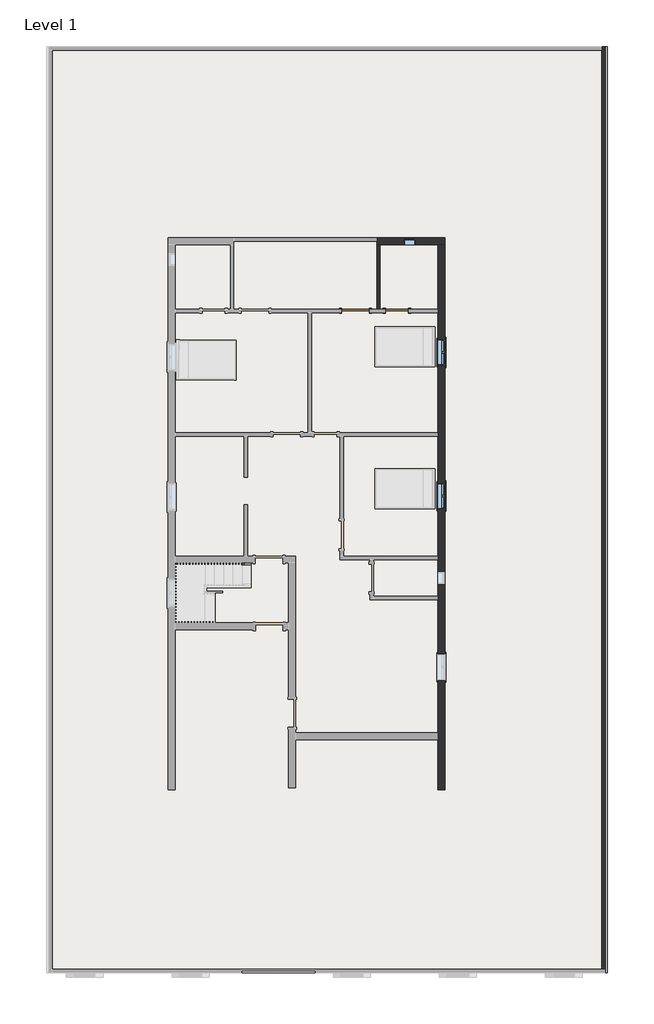
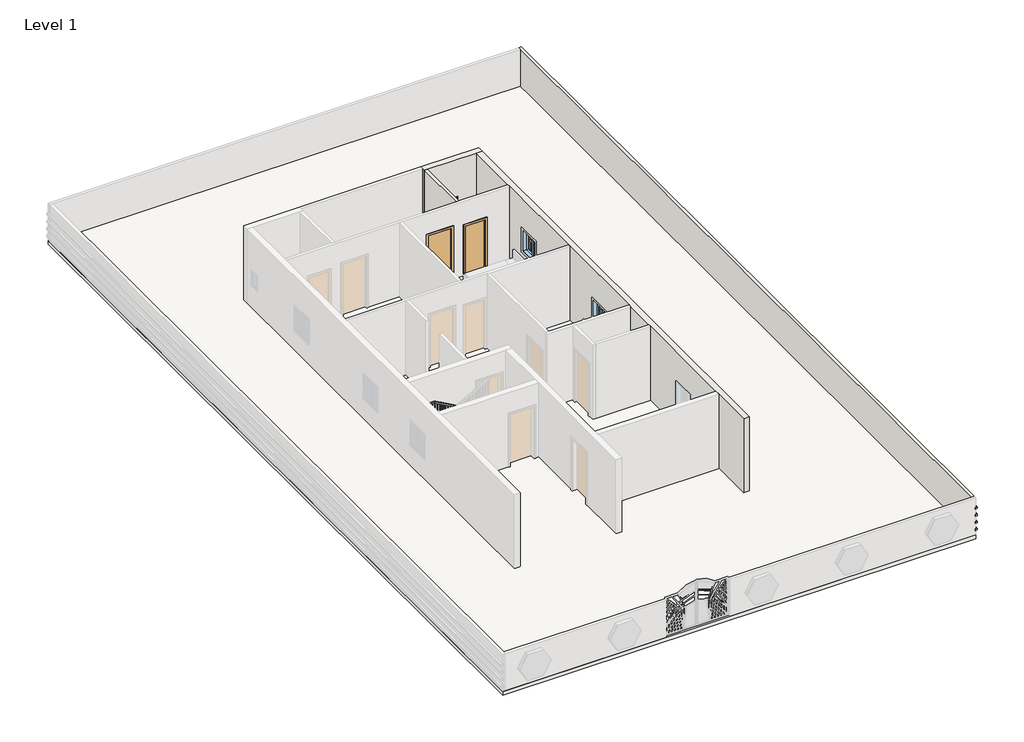
# One storey, part 2 of 3: 4 proxies, 4 walls, 3 windows, 2 doors, 1 railing, 1 slab.
"""IFC4 building model written with IfcOpenShell, lengths in millimetres."""

from ifc_helpers import new_model, si_unit, frame, origin, origin_with_axes, place, context, project, spatial, polyline, outline, extrude, faceted_brep, transform, mapped, element, save
from components import door_f2b275c1, door_e5f9f3c4, window_aa618e30, window_339605e1

model = new_model("IFC4")

# Units and contexts
model_context = context("Model", 3, world=origin())
ifc_project = project(units=[si_unit("LENGTHUNIT", "METRE", prefix="MILLI")], contexts=[model_context])

# Site, building, storey
site = spatial("IfcSite", under=ifc_project)
building = spatial("IfcBuilding", under=site)
storey = spatial("IfcBuildingStorey", under=building, Name="Level 1", Elevation=0.0)

# Proxies
placement = place(None, origin())
element("IfcBuildingElementProxy", 1, Name="Reveal", ObjectType="Reveal", at=placement, inside=storey, context=model_context, shape_type="SweptSolid", body=[
    extrude(outline(polyline([(8597.0265354, 16740.4715095), (8689.1015354, 16740.4715095), (8689.1015354, -13853.8284905), (8597.0265354, -13853.8284905), (8597.0265354, 16740.4715095)])), frame((0.0, 0.0, 1066.8), z_axis=(0.0, 0.0, 1.0), x_axis=(1.0, 0.0, 0.0)), (0.0, 0.0, 1.0), 67.7333333),
])
element("IfcBuildingElementProxy", 2, Name="Reveal", ObjectType="Reveal", at=placement, inside=storey, context=model_context, shape_type="SweptSolid", body=[
    extrude(outline(polyline([(8597.0265354, 16740.4715095), (8689.1015354, 16740.4715095), (8689.1015354, -13853.8284905), (8597.0265354, -13853.8284905), (8597.0265354, 16740.4715095)])), frame((0.0, 0.0, 772.755123), z_axis=(0.0, 0.0, 1.0), x_axis=(1.0, 0.0, 0.0)), (0.0, 0.0, 1.0), 67.7333333),
])
element("IfcBuildingElementProxy", 3, Name="Reveal", ObjectType="Reveal", at=placement, inside=storey, context=model_context, shape_type="SweptSolid", body=[
    extrude(outline(polyline([(8597.0265354, 16740.4715095), (8689.1015354, 16740.4715095), (8689.1015354, -13853.8284905), (8597.0265354, -13853.8284905), (8597.0265354, 16740.4715095)])), frame((0.0, 0.0, 478.710246), z_axis=(0.0, 0.0, 1.0), x_axis=(1.0, 0.0, 0.0)), (0.0, 0.0, 1.0), 67.7333333),
])
element("IfcBuildingElementProxy", 4, Name="Reveal", ObjectType="Reveal", at=placement, inside=storey, context=model_context, shape_type="SweptSolid", body=[
    extrude(outline(polyline([(8597.0265354, 16740.4715095), (8689.1015354, 16740.4715095), (8689.1015354, -13853.8284905), (8597.0265354, -13853.8284905), (8597.0265354, 16740.4715095)])), frame((0.0, 0.0, 184.6653689), z_axis=(0.0, 0.0, 1.0), x_axis=(1.0, 0.0, 0.0)), (0.0, 0.0, 1.0), 67.7333333),
])

# Doors
door_shape = door_f2b275c1(model_context)
element("IfcDoor", 5, ObjectType="Single-Flush : 30\" x 80\"", at=placement, inside=storey, context=model_context, shape_type="MappedRepresentation", body=[
    mapped(door_shape, transform((1735.6084916, 8007.7072267, 0.0), x_axis=(-1.0, 0.0, 0.0), y_axis=(0.0, -1.0, 0.0), z_axis=(0.0, 0.0, 1.0))),
])
door_2_shape = door_e5f9f3c4(model_context)
element("IfcDoor", 6, ObjectType="Single-Flush : 36\" x 84\"", at=placement, inside=storey, context=model_context, shape_type="MappedRepresentation", body=[
    mapped(door_2_shape, transform((364.0084916, 8007.7072267, 0.0), x_axis=(1.0, 0.0, 0.0), y_axis=(0.0, 1.0, 0.0), z_axis=(0.0, 0.0, 1.0))),
])

# Railing
element("IfcRailing", 7, ObjectType="Handrail - Rectangular", at=placement, inside=storey, context=model_context, shape_type="SolidModel", body=[
    faceted_brep([(-3084.0415084, -367.9427733, 1083.7333333), (-3084.0415084, -367.9427733, 1025.620221), (-3084.0415084, -317.1427733, 1025.620221), (-3084.0415084, -317.1427733, 1083.7333333), (-4608.0415084, -367.9427733, 1930.4), (-4621.2051106, -367.9427733, 1879.6), (-4621.2051106, -317.1427733, 1879.6), (-4608.0415084, -317.1427733, 1930.4), (-5547.8415084, -367.9427733, 1930.4), (-5547.8415084, -367.9427733, 1879.6), (-5598.6415084, -317.1427733, 1879.6), (-5598.6415084, -317.1427733, 1930.4), (-5547.8415084, -2247.5427733, 1930.4), (-5547.8415084, -2247.5427733, 1879.6), (-5598.6415084, -2298.3427733, 1879.6), (-5598.6415084, -2298.3427733, 1930.4), (-4912.8415084, -2247.5427733, 1930.4), (-4899.6779062, -2247.5427733, 1879.6), (-4899.6779062, -2298.3427733, 1879.6), (-4912.8415084, -2298.3427733, 1930.4), (-3084.0415084, -2247.5427733, 2946.4), (-3084.0415084, -2298.3427733, 2946.4), (-3084.0415084, -2298.3427733, 2888.2868876), (-3084.0415084, -2247.5427733, 2888.2868876)], [[[0, 1, 2, 3]], [[1, 0, 4, 5]], [[2, 1, 5, 6]], [[3, 2, 6, 7]], [[0, 3, 7, 4]], [[5, 4, 8, 9]], [[6, 5, 9, 10]], [[7, 6, 10, 11]], [[4, 7, 11, 8]], [[9, 8, 12, 13]], [[10, 9, 13, 14]], [[11, 10, 14, 15]], [[8, 11, 15, 12]], [[13, 12, 16, 17]], [[14, 13, 17, 18]], [[15, 14, 18, 19]], [[12, 15, 19, 16]], [[20, 21, 22, 23]], [[17, 16, 20, 23]], [[18, 17, 23, 22]], [[19, 18, 22, 21]], [[16, 19, 21, 20]]]),
    extrude(outline(polyline([(2865.3563321, -3125.3165084), (2854.7729988, -3144.3665084), (1862.6666667, -3144.3665084), (1862.6666667, -3125.3165084), (2865.3563321, -3125.3165084)])), frame((0.0, -2282.4677733, 0.0), z_axis=(0.0, 1.0, 0.0), x_axis=(0.0, 0.0, 1.0)), (0.0, 0.0, 1.0), 19.05),
    extrude(outline(polyline([(2808.9118876, -3226.9165084), (2798.3285543, -3245.9665084), (1862.6666667, -3245.9665084), (1862.6666667, -3226.9165084), (2808.9118876, -3226.9165084)])), frame((0.0, -2282.4677733, 0.0), z_axis=(0.0, 1.0, 0.0), x_axis=(0.0, 0.0, 1.0)), (0.0, 0.0, 1.0), 19.05),
    extrude(outline(polyline([(2752.4674432, -3328.5165084), (2741.8841099, -3347.5665084), (1862.6666667, -3347.5665084), (1862.6666667, -3328.5165084), (2752.4674432, -3328.5165084)])), frame((0.0, -2282.4677733, 0.0), z_axis=(0.0, 1.0, 0.0), x_axis=(0.0, 0.0, 1.0)), (0.0, 0.0, 1.0), 19.05),
    extrude(outline(polyline([(2696.0229988, -3430.1165084), (2685.4396654, -3449.1665084), (1693.3333333, -3449.1665084), (1693.3333333, -3430.1165084), (2696.0229988, -3430.1165084)])), frame((0.0, -2282.4677733, 0.0), z_axis=(0.0, 1.0, 0.0), x_axis=(0.0, 0.0, 1.0)), (0.0, 0.0, 1.0), 19.05),
    extrude(outline(polyline([(2639.5785543, -3531.7165084), (2628.995221, -3550.7665084), (1693.3333333, -3550.7665084), (1693.3333333, -3531.7165084), (2639.5785543, -3531.7165084)])), frame((0.0, -2282.4677733, 0.0), z_axis=(0.0, 1.0, 0.0), x_axis=(0.0, 0.0, 1.0)), (0.0, 0.0, 1.0), 19.05),
    extrude(outline(polyline([(2583.1341099, -3633.3165084), (2572.5507765, -3652.3665084), (1693.3333333, -3652.3665084), (1693.3333333, -3633.3165084), (2583.1341099, -3633.3165084)])), frame((0.0, -2282.4677733, 0.0), z_axis=(0.0, 1.0, 0.0), x_axis=(0.0, 0.0, 1.0)), (0.0, 0.0, 1.0), 19.05),
    extrude(outline(polyline([(2526.6896654, -3734.9165084), (2516.1063321, -3753.9665084), (1524.0, -3753.9665084), (1524.0, -3734.9165084), (2526.6896654, -3734.9165084)])), frame((0.0, -2282.4677733, 0.0), z_axis=(0.0, 1.0, 0.0), x_axis=(0.0, 0.0, 1.0)), (0.0, 0.0, 1.0), 19.05),
    extrude(outline(polyline([(2470.245221, -3836.5165084), (2459.6618876, -3855.5665084), (1524.0, -3855.5665084), (1524.0, -3836.5165084), (2470.245221, -3836.5165084)])), frame((0.0, -2282.4677733, 0.0), z_axis=(0.0, 1.0, 0.0), x_axis=(0.0, 0.0, 1.0)), (0.0, 0.0, 1.0), 19.05),
    extrude(outline(polyline([(2413.8007765, -3938.1165084), (2403.2174432, -3957.1665084), (1524.0, -3957.1665084), (1524.0, -3938.1165084), (2413.8007765, -3938.1165084)])), frame((0.0, -2282.4677733, 0.0), z_axis=(0.0, 1.0, 0.0), x_axis=(0.0, 0.0, 1.0)), (0.0, 0.0, 1.0), 19.05),
    extrude(outline(polyline([(2357.3563321, -4039.7165084), (2346.7729988, -4058.7665084), (1354.6666667, -4058.7665084), (1354.6666667, -4039.7165084), (2357.3563321, -4039.7165084)])), frame((0.0, -2282.4677733, 0.0), z_axis=(0.0, 1.0, 0.0), x_axis=(0.0, 0.0, 1.0)), (0.0, 0.0, 1.0), 19.05),
    extrude(outline(polyline([(2300.9118876, -4141.3165084), (2290.3285543, -4160.3665084), (1354.6666667, -4160.3665084), (1354.6666667, -4141.3165084), (2300.9118876, -4141.3165084)])), frame((0.0, -2282.4677733, 0.0), z_axis=(0.0, 1.0, 0.0), x_axis=(0.0, 0.0, 1.0)), (0.0, 0.0, 1.0), 19.05),
    extrude(outline(polyline([(2244.4674432, -4242.9165084), (2233.8841099, -4261.9665084), (1354.6666667, -4261.9665084), (1354.6666667, -4242.9165084), (2244.4674432, -4242.9165084)])), frame((0.0, -2282.4677733, 0.0), z_axis=(0.0, 1.0, 0.0), x_axis=(0.0, 0.0, 1.0)), (0.0, 0.0, 1.0), 19.05),
    extrude(outline(polyline([(2188.0229988, -4344.5165084), (2177.4396654, -4363.5665084), (1185.3333333, -4363.5665084), (1185.3333333, -4344.5165084), (2188.0229988, -4344.5165084)])), frame((0.0, -2282.4677733, 0.0), z_axis=(0.0, 1.0, 0.0), x_axis=(0.0, 0.0, 1.0)), (0.0, 0.0, 1.0), 19.05),
    extrude(outline(polyline([(2131.5785543, -4446.1165084), (2120.995221, -4465.1665084), (1185.3333333, -4465.1665084), (1185.3333333, -4446.1165084), (2131.5785543, -4446.1165084)])), frame((0.0, -2282.4677733, 0.0), z_axis=(0.0, 1.0, 0.0), x_axis=(0.0, 0.0, 1.0)), (0.0, 0.0, 1.0), 19.05),
    extrude(outline(polyline([(2075.1341099, -4547.7165084), (2064.5507765, -4566.7665084), (1185.3333333, -4566.7665084), (1185.3333333, -4547.7165084), (2075.1341099, -4547.7165084)])), frame((0.0, -2282.4677733, 0.0), z_axis=(0.0, 1.0, 0.0), x_axis=(0.0, 0.0, 1.0)), (0.0, 0.0, 1.0), 19.05),
    extrude(outline(polyline([(2018.6896654, -4649.3165084), (2008.1063321, -4668.3665084), (1016.0, -4668.3665084), (1016.0, -4649.3165084), (2018.6896654, -4649.3165084)])), frame((0.0, -2282.4677733, 0.0), z_axis=(0.0, 1.0, 0.0), x_axis=(0.0, 0.0, 1.0)), (0.0, 0.0, 1.0), 19.05),
    extrude(outline(polyline([(1962.245221, -4750.9165084), (1951.6618876, -4769.9665084), (1016.0, -4769.9665084), (1016.0, -4750.9165084), (1962.245221, -4750.9165084)])), frame((0.0, -2282.4677733, 0.0), z_axis=(0.0, 1.0, 0.0), x_axis=(0.0, 0.0, 1.0)), (0.0, 0.0, 1.0), 19.05),
    extrude(outline(polyline([(1905.8007765, -4852.5165084), (1895.2174432, -4871.5665084), (1016.0, -4871.5665084), (1016.0, -4852.5165084), (1905.8007765, -4852.5165084)])), frame((0.0, -2282.4677733, 0.0), z_axis=(0.0, 1.0, 0.0), x_axis=(0.0, 0.0, 1.0)), (0.0, 0.0, 1.0), 19.05),
    extrude(outline(polyline([(-4973.1665084, -2282.4677733), (-4973.1665084, -2263.4177733), (-4954.1165084, -2263.4177733), (-4954.1165084, -2282.4677733), (-4973.1665084, -2282.4677733)])), frame((0.0, 0.0, 1016.0), z_axis=(0.0, 0.0, 1.0), x_axis=(1.0, 0.0, 0.0)), (0.0, 0.0, 1.0), 863.6),
    extrude(outline(polyline([(-5074.7665084, -2282.4677733), (-5074.7665084, -2263.4177733), (-5055.7165084, -2263.4177733), (-5055.7165084, -2282.4677733), (-5074.7665084, -2282.4677733)])), frame((0.0, 0.0, 1016.0), z_axis=(0.0, 0.0, 1.0), x_axis=(1.0, 0.0, 0.0)), (0.0, 0.0, 1.0), 863.6),
    extrude(outline(polyline([(-5176.3665084, -2282.4677733), (-5176.3665084, -2263.4177733), (-5157.3165084, -2263.4177733), (-5157.3165084, -2282.4677733), (-5176.3665084, -2282.4677733)])), frame((0.0, 0.0, 1016.0), z_axis=(0.0, 0.0, 1.0), x_axis=(1.0, 0.0, 0.0)), (0.0, 0.0, 1.0), 863.6),
    extrude(outline(polyline([(-5277.9665084, -2282.4677733), (-5277.9665084, -2263.4177733), (-5258.9165084, -2263.4177733), (-5258.9165084, -2282.4677733), (-5277.9665084, -2282.4677733)])), frame((0.0, 0.0, 1016.0), z_axis=(0.0, 0.0, 1.0), x_axis=(1.0, 0.0, 0.0)), (0.0, 0.0, 1.0), 863.6),
    extrude(outline(polyline([(-5379.5665084, -2282.4677733), (-5379.5665084, -2263.4177733), (-5360.5165084, -2263.4177733), (-5360.5165084, -2282.4677733), (-5379.5665084, -2282.4677733)])), frame((0.0, 0.0, 1016.0), z_axis=(0.0, 0.0, 1.0), x_axis=(1.0, 0.0, 0.0)), (0.0, 0.0, 1.0), 863.6),
    extrude(outline(polyline([(-5481.1665084, -2282.4677733), (-5481.1665084, -2263.4177733), (-5462.1165084, -2263.4177733), (-5462.1165084, -2282.4677733), (-5481.1665084, -2282.4677733)])), frame((0.0, 0.0, 1016.0), z_axis=(0.0, 0.0, 1.0), x_axis=(1.0, 0.0, 0.0)), (0.0, 0.0, 1.0), 863.6),
    extrude(outline(polyline([(-5582.7665084, -2161.8177733), (-5563.7165084, -2161.8177733), (-5563.7165084, -2180.8677733), (-5582.7665084, -2180.8677733), (-5582.7665084, -2161.8177733)])), frame((0.0, 0.0, 1016.0), z_axis=(0.0, 0.0, 1.0), x_axis=(1.0, 0.0, 0.0)), (0.0, 0.0, 1.0), 863.6),
    extrude(outline(polyline([(-5582.7665084, -2060.2177733), (-5563.7165084, -2060.2177733), (-5563.7165084, -2079.2677733), (-5582.7665084, -2079.2677733), (-5582.7665084, -2060.2177733)])), frame((0.0, 0.0, 1016.0), z_axis=(0.0, 0.0, 1.0), x_axis=(1.0, 0.0, 0.0)), (0.0, 0.0, 1.0), 863.6),
    extrude(outline(polyline([(-5582.7665084, -1958.6177733), (-5563.7165084, -1958.6177733), (-5563.7165084, -1977.6677733), (-5582.7665084, -1977.6677733), (-5582.7665084, -1958.6177733)])), frame((0.0, 0.0, 1016.0), z_axis=(0.0, 0.0, 1.0), x_axis=(1.0, 0.0, 0.0)), (0.0, 0.0, 1.0), 863.6),
    extrude(outline(polyline([(-5582.7665084, -1857.0177733), (-5563.7165084, -1857.0177733), (-5563.7165084, -1876.0677733), (-5582.7665084, -1876.0677733), (-5582.7665084, -1857.0177733)])), frame((0.0, 0.0, 1016.0), z_axis=(0.0, 0.0, 1.0), x_axis=(1.0, 0.0, 0.0)), (0.0, 0.0, 1.0), 863.6),
    extrude(outline(polyline([(-5582.7665084, -1755.4177733), (-5563.7165084, -1755.4177733), (-5563.7165084, -1774.4677733), (-5582.7665084, -1774.4677733), (-5582.7665084, -1755.4177733)])), frame((0.0, 0.0, 1016.0), z_axis=(0.0, 0.0, 1.0), x_axis=(1.0, 0.0, 0.0)), (0.0, 0.0, 1.0), 863.6),
    extrude(outline(polyline([(-5582.7665084, -1653.8177733), (-5563.7165084, -1653.8177733), (-5563.7165084, -1672.8677733), (-5582.7665084, -1672.8677733), (-5582.7665084, -1653.8177733)])), frame((0.0, 0.0, 1016.0), z_axis=(0.0, 0.0, 1.0), x_axis=(1.0, 0.0, 0.0)), (0.0, 0.0, 1.0), 863.6),
    extrude(outline(polyline([(-5582.7665084, -1552.2177733), (-5563.7165084, -1552.2177733), (-5563.7165084, -1571.2677733), (-5582.7665084, -1571.2677733), (-5582.7665084, -1552.2177733)])), frame((0.0, 0.0, 1016.0), z_axis=(0.0, 0.0, 1.0), x_axis=(1.0, 0.0, 0.0)), (0.0, 0.0, 1.0), 863.6),
    extrude(outline(polyline([(-5582.7665084, -1450.6177733), (-5563.7165084, -1450.6177733), (-5563.7165084, -1469.6677733), (-5582.7665084, -1469.6677733), (-5582.7665084, -1450.6177733)])), frame((0.0, 0.0, 1016.0), z_axis=(0.0, 0.0, 1.0), x_axis=(1.0, 0.0, 0.0)), (0.0, 0.0, 1.0), 863.6),
    extrude(outline(polyline([(-5582.7665084, -1349.0177733), (-5563.7165084, -1349.0177733), (-5563.7165084, -1368.0677733), (-5582.7665084, -1368.0677733), (-5582.7665084, -1349.0177733)])), frame((0.0, 0.0, 1016.0), z_axis=(0.0, 0.0, 1.0), x_axis=(1.0, 0.0, 0.0)), (0.0, 0.0, 1.0), 863.6),
    extrude(outline(polyline([(-5582.7665084, -1247.4177733), (-5563.7165084, -1247.4177733), (-5563.7165084, -1266.4677733), (-5582.7665084, -1266.4677733), (-5582.7665084, -1247.4177733)])), frame((0.0, 0.0, 1016.0), z_axis=(0.0, 0.0, 1.0), x_axis=(1.0, 0.0, 0.0)), (0.0, 0.0, 1.0), 863.6),
    extrude(outline(polyline([(-5582.7665084, -1145.8177733), (-5563.7165084, -1145.8177733), (-5563.7165084, -1164.8677733), (-5582.7665084, -1164.8677733), (-5582.7665084, -1145.8177733)])), frame((0.0, 0.0, 1016.0), z_axis=(0.0, 0.0, 1.0), x_axis=(1.0, 0.0, 0.0)), (0.0, 0.0, 1.0), 863.6),
    extrude(outline(polyline([(-5582.7665084, -1044.2177733), (-5563.7165084, -1044.2177733), (-5563.7165084, -1063.2677733), (-5582.7665084, -1063.2677733), (-5582.7665084, -1044.2177733)])), frame((0.0, 0.0, 1016.0), z_axis=(0.0, 0.0, 1.0), x_axis=(1.0, 0.0, 0.0)), (0.0, 0.0, 1.0), 863.6),
    extrude(outline(polyline([(-5582.7665084, -942.6177733), (-5563.7165084, -942.6177733), (-5563.7165084, -961.6677733), (-5582.7665084, -961.6677733), (-5582.7665084, -942.6177733)])), frame((0.0, 0.0, 1016.0), z_axis=(0.0, 0.0, 1.0), x_axis=(1.0, 0.0, 0.0)), (0.0, 0.0, 1.0), 863.6),
    extrude(outline(polyline([(-5582.7665084, -841.0177733), (-5563.7165084, -841.0177733), (-5563.7165084, -860.0677733), (-5582.7665084, -860.0677733), (-5582.7665084, -841.0177733)])), frame((0.0, 0.0, 1016.0), z_axis=(0.0, 0.0, 1.0), x_axis=(1.0, 0.0, 0.0)), (0.0, 0.0, 1.0), 863.6),
    extrude(outline(polyline([(-5582.7665084, -739.4177733), (-5563.7165084, -739.4177733), (-5563.7165084, -758.4677733), (-5582.7665084, -758.4677733), (-5582.7665084, -739.4177733)])), frame((0.0, 0.0, 1016.0), z_axis=(0.0, 0.0, 1.0), x_axis=(1.0, 0.0, 0.0)), (0.0, 0.0, 1.0), 863.6),
    extrude(outline(polyline([(-5582.7665084, -637.8177733), (-5563.7165084, -637.8177733), (-5563.7165084, -656.8677733), (-5582.7665084, -656.8677733), (-5582.7665084, -637.8177733)])), frame((0.0, 0.0, 1016.0), z_axis=(0.0, 0.0, 1.0), x_axis=(1.0, 0.0, 0.0)), (0.0, 0.0, 1.0), 863.6),
    extrude(outline(polyline([(-5582.7665084, -536.2177733), (-5563.7165084, -536.2177733), (-5563.7165084, -555.2677733), (-5582.7665084, -555.2677733), (-5582.7665084, -536.2177733)])), frame((0.0, 0.0, 1016.0), z_axis=(0.0, 0.0, 1.0), x_axis=(1.0, 0.0, 0.0)), (0.0, 0.0, 1.0), 863.6),
    extrude(outline(polyline([(-5582.7665084, -434.6177733), (-5563.7165084, -434.6177733), (-5563.7165084, -453.6677733), (-5582.7665084, -453.6677733), (-5582.7665084, -434.6177733)])), frame((0.0, 0.0, 1016.0), z_axis=(0.0, 0.0, 1.0), x_axis=(1.0, 0.0, 0.0)), (0.0, 0.0, 1.0), 863.6),
    extrude(outline(polyline([(-5512.9165084, -333.0177733), (-5512.9165084, -352.0677733), (-5531.9665084, -352.0677733), (-5531.9665084, -333.0177733), (-5512.9165084, -333.0177733)])), frame((0.0, 0.0, 1016.0), z_axis=(0.0, 0.0, 1.0), x_axis=(1.0, 0.0, 0.0)), (0.0, 0.0, 1.0), 863.6),
    extrude(outline(polyline([(-5411.3165084, -333.0177733), (-5411.3165084, -352.0677733), (-5430.3665084, -352.0677733), (-5430.3665084, -333.0177733), (-5411.3165084, -333.0177733)])), frame((0.0, 0.0, 1016.0), z_axis=(0.0, 0.0, 1.0), x_axis=(1.0, 0.0, 0.0)), (0.0, 0.0, 1.0), 863.6),
    extrude(outline(polyline([(-5309.7165084, -333.0177733), (-5309.7165084, -352.0677733), (-5328.7665084, -352.0677733), (-5328.7665084, -333.0177733), (-5309.7165084, -333.0177733)])), frame((0.0, 0.0, 1016.0), z_axis=(0.0, 0.0, 1.0), x_axis=(1.0, 0.0, 0.0)), (0.0, 0.0, 1.0), 863.6),
    extrude(outline(polyline([(-5208.1165084, -333.0177733), (-5208.1165084, -352.0677733), (-5227.1665084, -352.0677733), (-5227.1665084, -333.0177733), (-5208.1165084, -333.0177733)])), frame((0.0, 0.0, 1016.0), z_axis=(0.0, 0.0, 1.0), x_axis=(1.0, 0.0, 0.0)), (0.0, 0.0, 1.0), 863.6),
    extrude(outline(polyline([(-5106.5165084, -333.0177733), (-5106.5165084, -352.0677733), (-5125.5665084, -352.0677733), (-5125.5665084, -333.0177733), (-5106.5165084, -333.0177733)])), frame((0.0, 0.0, 1016.0), z_axis=(0.0, 0.0, 1.0), x_axis=(1.0, 0.0, 0.0)), (0.0, 0.0, 1.0), 863.6),
    extrude(outline(polyline([(-5004.9165084, -333.0177733), (-5004.9165084, -352.0677733), (-5023.9665084, -352.0677733), (-5023.9665084, -333.0177733), (-5004.9165084, -333.0177733)])), frame((0.0, 0.0, 1016.0), z_axis=(0.0, 0.0, 1.0), x_axis=(1.0, 0.0, 0.0)), (0.0, 0.0, 1.0), 863.6),
    extrude(outline(polyline([(-4903.3165084, -333.0177733), (-4903.3165084, -352.0677733), (-4922.3665084, -352.0677733), (-4922.3665084, -333.0177733), (-4903.3165084, -333.0177733)])), frame((0.0, 0.0, 1016.0), z_axis=(0.0, 0.0, 1.0), x_axis=(1.0, 0.0, 0.0)), (0.0, 0.0, 1.0), 863.6),
    extrude(outline(polyline([(-4801.7165084, -333.0177733), (-4801.7165084, -352.0677733), (-4820.7665084, -352.0677733), (-4820.7665084, -333.0177733), (-4801.7165084, -333.0177733)])), frame((0.0, 0.0, 1016.0), z_axis=(0.0, 0.0, 1.0), x_axis=(1.0, 0.0, 0.0)), (0.0, 0.0, 1.0), 863.6),
    extrude(outline(polyline([(-4700.1165084, -333.0177733), (-4700.1165084, -352.0677733), (-4719.1665084, -352.0677733), (-4719.1665084, -333.0177733), (-4700.1165084, -333.0177733)])), frame((0.0, 0.0, 1016.0), z_axis=(0.0, 0.0, 1.0), x_axis=(1.0, 0.0, 0.0)), (0.0, 0.0, 1.0), 863.6),
    extrude(outline(polyline([(1866.995221, -4598.5165084), (1877.5785543, -4617.5665084), (1016.0, -4617.5665084), (1016.0, -4598.5165084), (1866.995221, -4598.5165084)])), frame((0.0, -352.0677733, 0.0), z_axis=(0.0, 1.0, 0.0), x_axis=(0.0, 0.0, 1.0)), (0.0, 0.0, 1.0), 19.05),
    extrude(outline(polyline([(1810.5507765, -4496.9165084), (1821.1341099, -4515.9665084), (846.6666667, -4515.9665084), (846.6666667, -4496.9165084), (1810.5507765, -4496.9165084)])), frame((0.0, -352.0677733, 0.0), z_axis=(0.0, 1.0, 0.0), x_axis=(0.0, 0.0, 1.0)), (0.0, 0.0, 1.0), 19.05),
    extrude(outline(polyline([(1754.1063321, -4395.3165084), (1764.6896654, -4414.3665084), (846.6666667, -4414.3665084), (846.6666667, -4395.3165084), (1754.1063321, -4395.3165084)])), frame((0.0, -352.0677733, 0.0), z_axis=(0.0, 1.0, 0.0), x_axis=(0.0, 0.0, 1.0)), (0.0, 0.0, 1.0), 19.05),
    extrude(outline(polyline([(1697.6618876, -4293.7165084), (1708.245221, -4312.7665084), (846.6666667, -4312.7665084), (846.6666667, -4293.7165084), (1697.6618876, -4293.7165084)])), frame((0.0, -352.0677733, 0.0), z_axis=(0.0, 1.0, 0.0), x_axis=(0.0, 0.0, 1.0)), (0.0, 0.0, 1.0), 19.05),
    extrude(outline(polyline([(1641.2174432, -4192.1165084), (1651.8007765, -4211.1665084), (677.3333333, -4211.1665084), (677.3333333, -4192.1165084), (1641.2174432, -4192.1165084)])), frame((0.0, -352.0677733, 0.0), z_axis=(0.0, 1.0, 0.0), x_axis=(0.0, 0.0, 1.0)), (0.0, 0.0, 1.0), 19.05),
    extrude(outline(polyline([(1584.7729988, -4090.5165084), (1595.3563321, -4109.5665084), (677.3333333, -4109.5665084), (677.3333333, -4090.5165084), (1584.7729988, -4090.5165084)])), frame((0.0, -352.0677733, 0.0), z_axis=(0.0, 1.0, 0.0), x_axis=(0.0, 0.0, 1.0)), (0.0, 0.0, 1.0), 19.05),
    extrude(outline(polyline([(1528.3285543, -3988.9165084), (1538.9118876, -4007.9665084), (677.3333333, -4007.9665084), (677.3333333, -3988.9165084), (1528.3285543, -3988.9165084)])), frame((0.0, -352.0677733, 0.0), z_axis=(0.0, 1.0, 0.0), x_axis=(0.0, 0.0, 1.0)), (0.0, 0.0, 1.0), 19.05),
    extrude(outline(polyline([(1471.8841099, -3887.3165084), (1482.4674432, -3906.3665084), (508.0, -3906.3665084), (508.0, -3887.3165084), (1471.8841099, -3887.3165084)])), frame((0.0, -352.0677733, 0.0), z_axis=(0.0, 1.0, 0.0), x_axis=(0.0, 0.0, 1.0)), (0.0, 0.0, 1.0), 19.05),
    extrude(outline(polyline([(1415.4396654, -3785.7165084), (1426.0229988, -3804.7665084), (508.0, -3804.7665084), (508.0, -3785.7165084), (1415.4396654, -3785.7165084)])), frame((0.0, -352.0677733, 0.0), z_axis=(0.0, 1.0, 0.0), x_axis=(0.0, 0.0, 1.0)), (0.0, 0.0, 1.0), 19.05),
    extrude(outline(polyline([(1358.995221, -3684.1165084), (1369.5785543, -3703.1665084), (508.0, -3703.1665084), (508.0, -3684.1165084), (1358.995221, -3684.1165084)])), frame((0.0, -352.0677733, 0.0), z_axis=(0.0, 1.0, 0.0), x_axis=(0.0, 0.0, 1.0)), (0.0, 0.0, 1.0), 19.05),
    extrude(outline(polyline([(1302.5507765, -3582.5165084), (1313.1341099, -3601.5665084), (338.6666667, -3601.5665084), (338.6666667, -3582.5165084), (1302.5507765, -3582.5165084)])), frame((0.0, -352.0677733, 0.0), z_axis=(0.0, 1.0, 0.0), x_axis=(0.0, 0.0, 1.0)), (0.0, 0.0, 1.0), 19.05),
    extrude(outline(polyline([(1246.1063321, -3480.9165084), (1256.6896654, -3499.9665084), (338.6666667, -3499.9665084), (338.6666667, -3480.9165084), (1246.1063321, -3480.9165084)])), frame((0.0, -352.0677733, 0.0), z_axis=(0.0, 1.0, 0.0), x_axis=(0.0, 0.0, 1.0)), (0.0, 0.0, 1.0), 19.05),
    extrude(outline(polyline([(1189.6618876, -3379.3165084), (1200.245221, -3398.3665084), (338.6666667, -3398.3665084), (338.6666667, -3379.3165084), (1189.6618876, -3379.3165084)])), frame((0.0, -352.0677733, 0.0), z_axis=(0.0, 1.0, 0.0), x_axis=(0.0, 0.0, 1.0)), (0.0, 0.0, 1.0), 19.05),
    extrude(outline(polyline([(1133.2174432, -3277.7165084), (1143.8007765, -3296.7665084), (169.3333333, -3296.7665084), (169.3333333, -3277.7165084), (1133.2174432, -3277.7165084)])), frame((0.0, -352.0677733, 0.0), z_axis=(0.0, 1.0, 0.0), x_axis=(0.0, 0.0, 1.0)), (0.0, 0.0, 1.0), 19.05),
    extrude(outline(polyline([(1076.7729988, -3176.1165084), (1087.3563321, -3195.1665084), (169.3333333, -3195.1665084), (169.3333333, -3176.1165084), (1076.7729988, -3176.1165084)])), frame((0.0, -352.0677733, 0.0), z_axis=(0.0, 1.0, 0.0), x_axis=(0.0, 0.0, 1.0)), (0.0, 0.0, 1.0), 19.05),
    extrude(outline(polyline([(-5582.7665084, -2263.4177733), (-5563.7165084, -2263.4177733), (-5563.7165084, -2282.4677733), (-5582.7665084, -2282.4677733), (-5582.7665084, -2263.4177733)])), frame((0.0, 0.0, 1016.0), z_axis=(0.0, 0.0, 1.0), x_axis=(1.0, 0.0, 0.0)), (0.0, 0.0, 1.0), 863.6),
    extrude(outline(polyline([(-5563.7165084, -333.0177733), (-5563.7165084, -352.0677733), (-5582.7665084, -352.0677733), (-5582.7665084, -333.0177733), (-5563.7165084, -333.0177733)])), frame((0.0, 0.0, 1016.0), z_axis=(0.0, 0.0, 1.0), x_axis=(1.0, 0.0, 0.0)), (0.0, 0.0, 1.0), 863.6),
    extrude(outline(polyline([(2888.2868876, -3084.0415084), (2877.7035543, -3103.0915084), (1862.6666667, -3103.0915084), (1862.6666667, -3084.0415084), (2888.2868876, -3084.0415084)])), frame((0.0, -2282.4677733, 0.0), z_axis=(0.0, 1.0, 0.0), x_axis=(0.0, 0.0, 1.0)), (0.0, 0.0, 1.0), 19.05),
    extrude(outline(polyline([(1025.620221, -3084.0415084), (1036.2035543, -3103.0915084), (169.3333333, -3103.0915084), (169.3333333, -3084.0415084), (1025.620221, -3084.0415084)])), frame((0.0, -352.0677733, 0.0), z_axis=(0.0, 1.0, 0.0), x_axis=(0.0, 0.0, 1.0)), (0.0, 0.0, 1.0), 19.05),
])

# Slab
element("IfcSlab", 8, ObjectType="Generic - 12\"", at=placement, inside=storey, context=model_context, shape_type="SweptSolid", body=[
    extrude(outline(polyline([(8622.4265354, 16740.4715095), (8622.4265354, -13853.8284905), (-9779.8734646, -13853.8284905), (-9779.8734646, 16740.4715095), (8622.4265354, 16740.4715095)])), frame((0.0, 0.0, -152.4), z_axis=(0.0, 0.0, 1.0), x_axis=(1.0, 0.0, 0.0)), (0.0, 0.0, 1.0), 152.4),
])

# Walls
element("IfcWall", 9, ObjectType="WALL4.5\"", at=placement, inside=storey, context=model_context, shape_type="SweptSolid", body=[
    extrude(outline(polyline([(1068.8584916, 8064.8572267), (1068.8584916, 10198.4572267), (1183.1584916, 10198.4572267), (1183.1584916, 8064.8572267), (1068.8584916, 8064.8572267)])), origin_with_axes(), (0.0, 0.0, 1.0), 3048.0),
])
element("IfcWall", 10, ObjectType="WALL4.5\"", at=placement, inside=storey, context=model_context, shape_type="Brep", body=[
    faceted_brep([(8508.1265354, 16740.4715095, 0.0), (8508.1265354, 16626.1715095, 0.0), (8508.1265354, -13739.5284905, 0.0), (8508.1265354, -13739.5284905, 1524.0), (8508.1265354, 16626.1715095, 1524.0), (8508.1265354, 16740.4715095, 1524.0), (8622.4265354, -13739.5284905, 0.0), (8622.4265354, 16740.4715095, 0.0), (8622.4265354, 16740.4715095, 184.6653689), (8622.4265354, -13739.5284905, 184.6653689), (8622.4265354, 16740.4715095, 1524.0), (8622.4265354, -13739.5284905, 1524.0), (8622.4265354, -13739.5284905, 1134.5333333), (8622.4265354, 16740.4715095, 1134.5333333), (8622.4265354, 16740.4715095, 1066.8), (8622.4265354, -13739.5284905, 1066.8), (8622.4265354, -13739.5284905, 840.4884563), (8622.4265354, 16740.4715095, 840.4884563), (8622.4265354, 16740.4715095, 772.755123), (8622.4265354, -13739.5284905, 772.755123), (8622.4265354, -13739.5284905, 546.4435793), (8622.4265354, 16740.4715095, 546.4435793), (8622.4265354, 16740.4715095, 478.710246), (8622.4265354, -13739.5284905, 478.710246), (8622.4265354, -13739.5284905, 252.3987023), (8622.4265354, 16740.4715095, 252.3987023), (8597.0265354, 16740.4715095, 1134.5333333), (8597.0265354, 16740.4715095, 1066.8), (8597.0265354, 16740.4715095, 840.4884563), (8597.0265354, 16740.4715095, 772.755123), (8597.0265354, 16740.4715095, 546.4435793), (8597.0265354, 16740.4715095, 478.710246), (8597.0265354, 16740.4715095, 252.3987023), (8597.0265354, 16740.4715095, 184.6653689), (8597.0265354, -13739.5284905, 184.6653689), (8597.0265354, -13739.5284905, 252.3987023), (8597.0265354, -13739.5284905, 478.710246), (8597.0265354, -13739.5284905, 546.4435793), (8597.0265354, -13739.5284905, 772.755123), (8597.0265354, -13739.5284905, 840.4884563), (8597.0265354, -13739.5284905, 1066.8), (8597.0265354, -13739.5284905, 1134.5333333)], [[[0, 1, 2, 3, 4, 5]], [[6, 7, 8, 9]], [[10, 11, 12, 13]], [[14, 15, 16, 17]], [[18, 19, 20, 21]], [[22, 23, 24, 25]], [[2, 1, 0, 7, 6]], [[5, 4, 3, 11, 10]], [[0, 5, 10, 13, 26, 27, 14, 17, 28, 29, 18, 21, 30, 31, 22, 25, 32, 33, 8, 7]], [[3, 2, 6, 9, 34, 35, 24, 23, 36, 37, 20, 19, 38, 39, 16, 15, 40, 41, 12, 11]], [[41, 26, 13, 12]], [[27, 40, 15, 14]], [[26, 41, 40, 27]], [[39, 28, 17, 16]], [[29, 38, 19, 18]], [[28, 39, 38, 29]], [[37, 30, 21, 20]], [[31, 36, 23, 22]], [[30, 37, 36, 31]], [[35, 32, 25, 24]], [[33, 34, 9, 8]], [[32, 35, 34, 33]]]),
])
element("IfcWall", 11, ObjectType="WALL9\"", at=placement, inside=storey, context=model_context, shape_type="Brep", body=[
    faceted_brep([(1068.8584916, 10198.4572267, 0.0), (1183.1584916, 10198.4572267, 0.0), (3088.1584916, 10198.4572267, 0.0), (3316.7584916, 10198.4572267, 0.0), (3316.7584916, 10198.4572267, 3048.0), (3088.1584916, 10198.4572267, 3048.0), (1183.1584916, 10198.4572267, 3048.0), (1068.8584916, 10198.4572267, 3048.0), (2367.4334916, 10198.4572267, 1524.0), (2367.4334916, 10198.4572267, 914.4), (1961.0334916, 10198.4572267, 914.4), (1961.0334916, 10198.4572267, 1524.0), (1068.8584916, 10427.0572267, 0.0), (1068.8584916, 10427.0572267, 3048.0), (3316.7584916, 10427.0572267, 3048.0), (3316.7584916, 10427.0572267, 0.0), (2367.4334916, 10427.0572267, 1524.0), (1961.0334916, 10427.0572267, 1524.0), (1961.0334916, 10427.0572267, 914.4), (2367.4334916, 10427.0572267, 914.4), (1068.8584916, 10312.7572267, 0.0), (1068.8584916, 10312.7572267, 3048.0)], [[[0, 1, 2, 3, 4, 5, 6, 7], [8, 9, 10, 11]], [[12, 13, 14, 15], [16, 17, 18, 19]], [[3, 2, 1, 0, 20, 12, 15]], [[4, 3, 15, 14]], [[0, 7, 21, 13, 12, 20]], [[9, 8, 16, 19]], [[10, 9, 19, 18]], [[11, 10, 18, 17]], [[8, 11, 17, 16]], [[7, 6, 5, 4, 14, 13, 21]]]),
])
element("IfcWall", 12, ObjectType="WALL9\"", at=placement, inside=storey, context=model_context, shape_type="Brep", body=[
    faceted_brep([(3088.1584916, 10198.4572267, 0.0), (3088.1584916, 8064.8572267, 0.0), (3088.1584916, 7950.5572267, 0.0), (3088.1584916, 3988.1572267, 0.0), (3088.1584916, 3873.8572267, 0.0), (3088.1584916, -88.5427733, 0.0), (3088.1584916, -202.8427733, 0.0), (3088.1584916, -1422.0427733, 0.0), (3088.1584916, -1536.3427733, 0.0), (3088.1584916, -5930.5427733, 0.0), (3088.1584916, -6159.1427733, 0.0), (3088.1584916, -7803.7927733, 0.0), (3088.1584916, -7803.7927733, 3048.0), (3088.1584916, -6159.1427733, 3048.0), (3088.1584916, -5930.5427733, 3048.0), (3088.1584916, -1536.3427733, 3048.0), (3088.1584916, -1422.0427733, 3048.0), (3088.1584916, -202.8427733, 3048.0), (3088.1584916, -88.5427733, 3048.0), (3088.1584916, 3873.8572267, 3048.0), (3088.1584916, 3988.1572267, 3048.0), (3088.1584916, 7950.5572267, 3048.0), (3088.1584916, 8064.8572267, 3048.0), (3088.1584916, 10198.4572267, 3048.0), (3088.1584916, -1015.6427733, 1524.0), (3088.1584916, -1015.6427733, 914.4), (3088.1584916, -609.2427733, 914.4), (3088.1584916, -609.2427733, 1524.0), (3088.1584916, 6204.3072267, 1828.8), (3088.1584916, 6204.3072267, 914.4), (3088.1584916, 7067.9072267, 914.4), (3088.1584916, 7067.9072267, 1828.8), (3088.1584916, 1460.8572267, 1828.8), (3088.1584916, 1460.8572267, 914.4), (3088.1584916, 2324.4572267, 914.4), (3088.1584916, 2324.4572267, 1828.8), (3088.1584916, -4193.8177733, 1828.8), (3088.1584916, -4193.8177733, 914.4), (3088.1584916, -3330.2177733, 914.4), (3088.1584916, -3330.2177733, 1828.8), (3316.7584916, 10198.4572267, 0.0), (3316.7584916, 10198.4572267, 3048.0), (3316.7584916, -7803.7927733, 3048.0), (3316.7584916, -7803.7927733, 0.0), (3316.7584916, -1015.6427733, 1524.0), (3316.7584916, -609.2427733, 1524.0), (3316.7584916, -609.2427733, 914.4), (3316.7584916, -1015.6427733, 914.4), (3316.7584916, 6204.3072267, 1828.8), (3316.7584916, 7067.9072267, 1828.8), (3316.7584916, 7067.9072267, 914.4), (3316.7584916, 6204.3072267, 914.4), (3316.7584916, 1460.8572267, 1828.8), (3316.7584916, 2324.4572267, 1828.8), (3316.7584916, 2324.4572267, 914.4), (3316.7584916, 1460.8572267, 914.4), (3316.7584916, -4193.8177733, 1828.8), (3316.7584916, -3330.2177733, 1828.8), (3316.7584916, -3330.2177733, 914.4), (3316.7584916, -4193.8177733, 914.4)], [[[0, 1, 2, 3, 4, 5, 6, 7, 8, 9, 10, 11, 12, 13, 14, 15, 16, 17, 18, 19, 20, 21, 22, 23], [24, 25, 26, 27], [28, 29, 30, 31], [32, 33, 34, 35], [36, 37, 38, 39]], [[40, 41, 42, 43], [44, 45, 46, 47], [48, 49, 50, 51], [52, 53, 54, 55], [56, 57, 58, 59]], [[11, 10, 9, 8, 7, 6, 5, 4, 3, 2, 1, 0, 40, 43]], [[12, 11, 43, 42]], [[0, 23, 41, 40]], [[25, 24, 44, 47]], [[26, 25, 47, 46]], [[27, 26, 46, 45]], [[24, 27, 45, 44]], [[29, 28, 48, 51]], [[30, 29, 51, 50]], [[31, 30, 50, 49]], [[28, 31, 49, 48]], [[33, 32, 52, 55]], [[34, 33, 55, 54]], [[35, 34, 54, 53]], [[32, 35, 53, 52]], [[37, 36, 56, 59]], [[38, 37, 59, 58]], [[39, 38, 58, 57]], [[36, 39, 57, 56]], [[23, 22, 21, 20, 19, 18, 17, 16, 15, 14, 13, 12, 42, 41]]]),
])

# Windows
window_shape = window_aa618e30(model_context)
element("IfcWindow", 13, ObjectType="Fixed : 16\" x 24\"", at=placement, inside=storey, context=model_context, shape_type="MappedRepresentation", body=[
    mapped(window_shape, transform((2202.3334916, 10312.7572267, 0.0), x_axis=(1.0, 0.0, 0.0), y_axis=(0.0, 1.0, 0.0), z_axis=(0.0, 0.0, 1.0))),
])
window_2_shape = window_339605e1(model_context)
element("IfcWindow", 14, ObjectType="Window-Casement-Double : 34\" x 36\"", at=placement, inside=storey, context=model_context, shape_type="MappedRepresentation", body=[
    mapped(window_2_shape, transform((3202.4584916, 6636.1072267, 0.0), x_axis=(0.0, -1.0, 0.0), y_axis=(1.0, 0.0, 0.0), z_axis=(0.0, 0.0, 1.0))),
])
element("IfcWindow", 15, ObjectType="Window-Casement-Double : 34\" x 36\"", at=placement, inside=storey, context=model_context, shape_type="MappedRepresentation", body=[
    mapped(window_2_shape, transform((3202.4584916, 1892.6572267, 0.0), x_axis=(0.0, -1.0, 0.0), y_axis=(1.0, 0.0, 0.0), z_axis=(0.0, 0.0, 1.0))),
])

save(model, "model.ifc")

# Revit data of these elements
# Type "Single-Flush : 30\" x 80\""
#   Type Mark = "5"
#   Construction Type Id = "MDOOR"
#   Assembly Code = "C1020"
#   Analytic Construction = "Metal"
#   Thickness = 0' - 2"
#   Heat Transfer Coefficient (U) = 0.651978 BTU/(h·ft²·°F)
#   Height = 6' - 8"
#   Trim Projection Ext = 0' - 1"
#   Trim Projection Int = 0' - 1"
#   Trim Width = 0' - 3"
#   Width = 2' - 6"
#   Define Thermal Properties by = 1
#   Define Thermal Properties by = 1
#   Door Material = Door - Panel
#   Frame Material = Door - Frame
#   Visual Light Transmittance = 0
#   Solar Heat Gain Coefficient = 0
#   Function = (empty or 0)
#   Wall Closure = (empty or 0)
# Type "Single-Flush : 36\" x 84\""
#   Type Mark = "1"
#   Construction Type Id = "MDOOR"
#   Assembly Code = "C1020"
#   Analytic Construction = "Metal"
#   Thickness = 0' - 2"
#   Heat Transfer Coefficient (U) = 0.651978 BTU/(h·ft²·°F)
#   Height = 7' - 0"
#   Trim Projection Ext = 0' - 1"
#   Trim Projection Int = 0' - 1"
#   Trim Width = 0' - 3"
#   Width = 3' - 0"
#   Define Thermal Properties by = 1
#   Define Thermal Properties by = 1
#   Door Material = Door - Panel
#   Frame Material = Door - Frame
#   Visual Light Transmittance = 0
#   Solar Heat Gain Coefficient = 0
#   Function = (empty or 0)
#   Wall Closure = (empty or 0)
# Type "Handrail - Rectangular"
#   Assembly Code = "C2010400"
#   built-in parameter 1008612 = 0.0416667 (stored number, unit not read)
#   built-in parameter 1008611 = 0.0416667 (stored number, unit not read)
#   built-in parameter 1008609 = 0.333333 (stored number, unit not read)
#   built-in parameter 1008604 = 0.166667 (stored number, unit not read)
#   built-in parameter 1008603 = 0.166667 (stored number, unit not read)
#   Railing Height = 3' - 0"
#   built-in parameter 1008630 = 2
#   built-in parameter 1008610 = 2
#   built-in parameter 1008618 = Baluster - Square : 3/4"
# Type "Generic - 12\""
#   Assembly Code = "B1010"
#   Function = 0
#   Layers, outside or top first: 0' - 6" no material (function 1)
# Type "WALL4.5\""
#   Assembly Code = "B2010"
#   Layers, outside or top first: 0' - 4 1/2" no material (function 1)
# Type "WALL9\""
#   Assembly Code = "B2010"
#   Layers, outside or top first: 0' - 9" no material (function 1)
# Type "Fixed : 16\" x 24\""
#   Type Mark = "4"
#   Construction Type Id = "GSP4R"
#   Assembly Code = "B2020100"
#   Analytic Construction = "1/8 in Pilkington single glazing"
#   Visual Light Transmittance = 0.9
#   Solar Heat Gain Coefficient = 0.78
#   Heat Transfer Coefficient (U) = 0.6496 BTU/(h·ft²·°F)
#   Height = 2' - 0"
#   Default Sill Height = 3' - 0"
#   Width = 1' - 4"
#   Window Inset = 0' - 0 3/4"
#   Define Thermal Properties by = 1
#   Define Thermal Properties by = 1
#   Glass Pane Material = Glass
#   Sash Material = Sash
#   Wall Closure = (empty or 0)
# Type "Window-Casement-Double : 34\" x 36\""
#   Type Mark = "14"
#   Fire Rating = "0.5h"
#   Assembly Code = "B2020100"
#   Analytic Construction = "Double glazing - domestic"
#   Frame Extension [instance default] = 0' - 0 1/4"
#   Window Inset [instance default] = 0' - 0"
#   Wall Thickness [instance default] = 0' - 6"
#   Interior Wall Closure [instance default] = 0' - 2 1/4"
#   Half Width = 1' - 5"
#   Visual Light Transmittance = 0.81
#   Thermal Resistance (R) = 1.8146 (h·ft²·°F)/BTU
#   Solar Heat Gain Coefficient = 0.76
#   Rough Width = 2' - 10 1/2"
#   Rough Height = 3' - 0 1/2"
#   Height = 3' - 0"
#   Heat Transfer Coefficient (U) = 0.5511 BTU/(h·ft²·°F)
#   Exterior Wall Closure [instance default] = 0' - 1 1/4"
#   Extension Jamb [instance default] = 0' - 2 1/4"
#   Default Sill Height = 3' - 0"
#   Width = 2' - 10"
#   Define Thermal Properties by = 0
#   Muntin Visibility = yes
#   Interior Trim Visibility [instance default] = yes
#   Exterior Trim Visibility [instance default] = yes
#   Extension Jamb Visibility [instance default] = yes
#   Interior Trim Material = Wood - Stained
#   Muntin Pattern = Muntin Pattern_2x2 : Muntin Pattern_2x2
#   Interior Trim = Trim-Window-Interior-Flat : Picture Frame
#   Interior Frame Material = Wood - Stained
#   Glass Panel Material = Glass
#   Exterior Trim Material = Clad - White
#   Exterior Trim = Trim-Window-Exterior-Flat : with Sill
#   Exterior Frame Material = Clad - White
#   Wall Closure = (empty or 0)
# Element 5 (IfcDoor, "Single-Flush : 30\" x 80\"")
#   Phase Created = New Construction
#   Materials on its faces: "Door - Frame", "Door - Panel"
# Element 6 (IfcDoor, "Single-Flush : 36\" x 84\"")
#   Phase Created = New Construction
#   Materials on its faces: "Door - Frame", "Door - Panel"
# Element 7 (IfcRailing, "Handrail - Rectangular")
#   Phase Created = New Construction
# Element 8 (IfcSlab, "Generic - 12\"")
#   Height Offset From Level = 0' - 0"
#   Phase Created = New Construction
#   Materials on its faces: "Default Floor"
# Element 9 (IfcWall, "WALL4.5\"")
#   Top Offset = 0' - 0"
#   Base Offset = 0' - 0"
#   Unconnected Height = 10' - 0"
#   wall height = 10' - 0"
#   Phase Created = New Construction
#   Base Constraint = Level 1
#   Materials on its faces: "Default Wall", "Wood Planks"
# Element 10 (IfcWall, "WALL4.5\"")
#   Top Offset = 0' - 0"
#   Base Offset = 0' - 0"
#   Unconnected Height = 5' - 0"
#   wall height = 5' - 0"
#   Phase Created = New Construction
#   Base Constraint = Level 1
#   Materials on its faces: "Default Wall", "Door - Frame"
# Elements 11, 12 (IfcWall, "WALL9\"")
#   Top Offset = 0' - 0"
#   Base Offset = 0' - 0"
#   Unconnected Height = 10' - 0"
#   wall height = 10' - 0"
#   Phase Created = New Construction
#   Base Constraint = Level 1
#   Materials on its faces: "Default Wall", "Wood Planks"
# Element 13 (IfcWindow, "Fixed : 16\" x 24\"")
#   Mark = "2"
#   Phase Created = New Construction
#   Materials on its faces: "Sash", "Glass"
# Element 14 (IfcWindow, "Window-Casement-Double : 34\" x 36\"")
#   Mark = "4"
#   Window Inset = 0' - 0"
#   Interior Wall Closure = 0' - 2 1/4"
#   Frame Extension = 0' - 0 1/4"
#   Exterior Wall Closure = 0' - 1 1/4"
#   Interior Trim Visibility = yes
#   Exterior Trim Visibility = yes
#   Phase Created = New Construction
#   Materials on its faces: "Wood - Stained", "Glass", "Clad - White"
# Element 15 (IfcWindow, "Window-Casement-Double : 34\" x 36\"")
#   Mark = "5"
#   Window Inset = 0' - 0"
#   Interior Wall Closure = 0' - 2 1/4"
#   Frame Extension = 0' - 0 1/4"
#   Exterior Wall Closure = 0' - 1 1/4"
#   Interior Trim Visibility = yes
#   Exterior Trim Visibility = yes
#   Phase Created = New Construction
#   Materials on its faces: "Wood - Stained", "Glass", "Clad - White"
# Materials
#   "Door - Panel": class "Wood", colour RGB 210 159 95, transparency 0, Cost = 0
#   "Door - Frame": colour RGB 118 70 51, transparency 0, Cost = 0
#   "Glass": class "Glass", colour RGB 0 128 192, transparency 0.75, Description = "Soda Lime Glass", Cost = 0
#   "Sash": class "Wood", colour RGB 224 178 126, transparency 0, Cost = 0
#   "Wood - Stained": class "Wood", colour RGB 224 178 126, transparency 0, Cost = 0
#   "Clad - White": class "Wood", colour RGB 242 242 238, transparency 0, Cost = 0
#   "Default Floor": colour RGB 128 128 128, transparency 0, Cost = 0
#   "Default Wall": colour RGB 128 128 128, transparency 0, Cost = 0
#   "Wood Planks": class "Wood", colour RGB 193 160 115, transparency 0, Description = "Physical material.", Cost = 0
